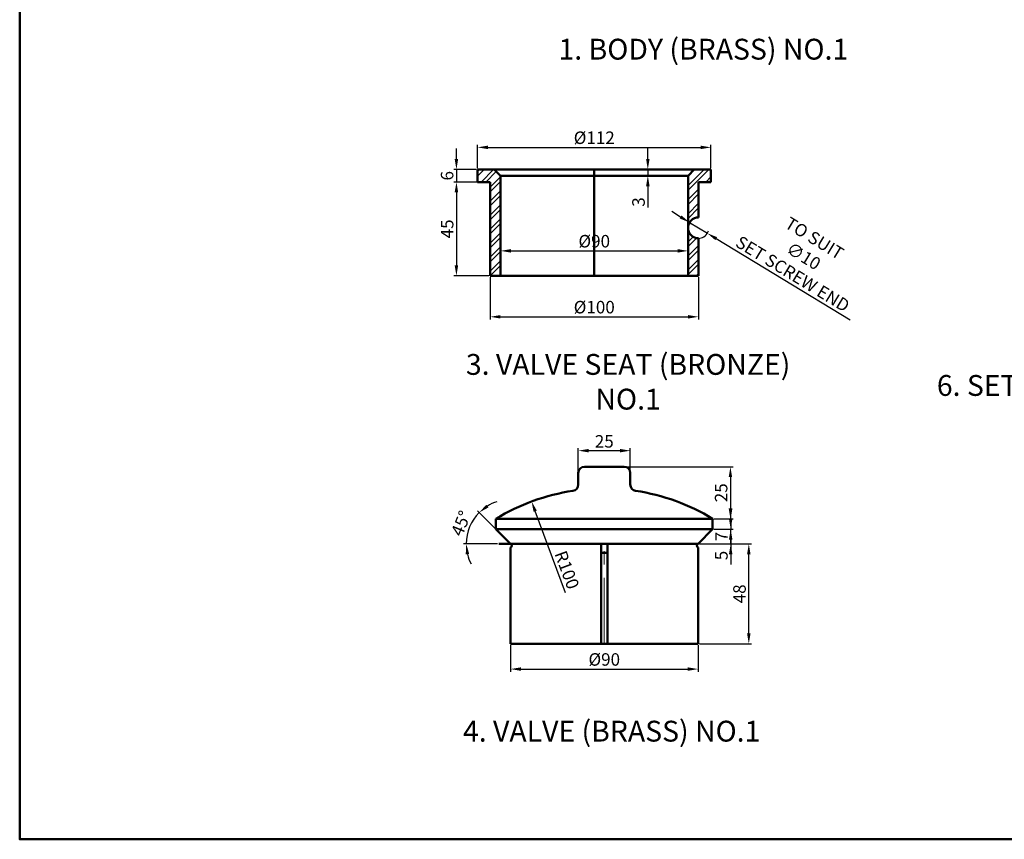
# Model space of a CAD drawing. Units: millimetres. Extents: x -907 to -46, y -312 to 510.
# Tile 1 of 3: x -907 to -434, y -312 to 81. Entities that reach past the tile are written whole.
import ezdxf

# ---------------------------------------------------------------- set-up
doc = ezdxf.new("R2010")
doc.units = ezdxf.units.MM
doc.linetypes.add('CENTER', pattern=[50.8, 31.75, -6.35, 6.35, -6.35])
for name, color, linetype, lineweight in [('M-CNTR', 1, 'CENTER', 18), ('M-DIMS', 2, 'Continuous', 25), ('M-HATC', 8, 'Continuous', 18), ('M-OUTL', 7, 'Continuous', 50), ('M-TEXT', 3, 'Continuous', 25), ('M-TTLB', 7, 'Continuous', 50)]:
    doc.layers.add(name, color=color, linetype=linetype, lineweight=lineweight)
doc.styles.get("Standard").update_dxf_attribs({"font": 'arial.ttf'})
doc.dimstyles.new('ISO-25', dxfattribs={"dimtxt": 6, "dimasz": 5, "dimexe": 1.25, "dimexo": 0.625, "dimtad": 1, "dimtxsty": 'Standard', "dimcen": 2.5, "dimadec": 0, "dimazin": 0, "dimtfac": 1, "dimtmove": 0, "dimatfit": 3, "dimfxl": 1, "dimarcsym": 0})

# ---------------------------------------------------------------- blocks, each defined once
blk = doc.blocks.new('*D24')
at = {"layer": 'Defpoints', "color": 0, "transparency": 16777216}
for p in [(-681.22, -41.73), (-581.22, -41.73), (-581.22, -61.42)]:
    blk.add_point(p, dxfattribs=at)
at = {"layer": 'M-DIMS', "color": 0, "lineweight": -2, "transparency": 16777216}
for p, q in [((-681.22, -42.36), (-681.22, -62.67)), ((-581.22, -42.36), (-581.22, -62.67)), ((-676.22, -61.42), (-586.22, -61.42))]:
    blk.add_line(p, q, dxfattribs=at)
at = {"layer": 'M-DIMS', "color": 0, "transparency": 16777216}
for points in [[(-676.22, -60.58), (-676.22, -62.25), (-681.22, -61.42)], [(-586.22, -60.58), (-586.22, -62.25), (-581.22, -61.42)]]:
    blk.add_solid(points, dxfattribs=at)
at = {"layer": 'M-DIMS', "color": 0, "transparency": 16777216, "insert": (-631.22, -57.56), "char_height": 6, "attachment_point": 5}
blk.add_mtext('%%C100', dxfattribs=at)
blk = doc.blocks.new('*D25')
at = {"layer": 'Defpoints', "color": 0, "transparency": 16777216}
for p in [(-676.22, -21.78), (-586.22, -21.78), (-586.22, -29.78)]:
    blk.add_point(p, dxfattribs=at)
at = {"layer": 'M-DIMS', "color": 0, "lineweight": -2, "transparency": 16777216}
for p, q in [((-676.22, -22.41), (-676.22, -31.03)), ((-586.22, -22.41), (-586.22, -31.03)), ((-671.22, -29.78), (-591.22, -29.78))]:
    blk.add_line(p, q, dxfattribs=at)
at = {"layer": 'M-DIMS', "color": 0, "transparency": 16777216}
for points in [[(-671.22, -28.94), (-671.22, -30.61), (-676.22, -29.78)], [(-591.22, -28.94), (-591.22, -30.61), (-586.22, -29.78)]]:
    blk.add_solid(points, dxfattribs=at)
at = {"layer": 'M-DIMS', "color": 0, "transparency": 16777216, "insert": (-631.22, -25.92), "char_height": 6, "attachment_point": 5}
blk.add_mtext('%%C90', dxfattribs=at)
blk = doc.blocks.new('*D26')
at = {"layer": 'Defpoints', "color": 0, "transparency": 16777216}
for p in [(-606.21, 9.27), (-606.21, 6.27), (-605.51, 6.27)]:
    blk.add_point(p, dxfattribs=at)
at = {"layer": 'M-DIMS', "color": 0, "lineweight": -2, "transparency": 16777216}
for p, q in [((-605.51, 14.27), (-605.51, 19.27)), ((-605.59, 9.27), (-604.26, 9.27)), ((-605.59, 6.27), (-604.26, 6.27)), ((-605.51, 9.27), (-605.51, 6.27)), ((-605.51, 1.27), (-605.51, -8.91))]:
    blk.add_line(p, q, dxfattribs=at)
at = {"layer": 'M-DIMS', "color": 0, "transparency": 16777216}
for points in [[(-606.34, 14.27), (-604.68, 14.27), (-605.51, 9.27)], [(-606.34, 1.27), (-604.68, 1.27), (-605.51, 6.27)]]:
    blk.add_solid(points, dxfattribs=at)
at = {"layer": 'M-DIMS', "color": 0, "transparency": 16777216, "insert": (-609.2, -6.32), "char_height": 6, "attachment_point": 5, "rotation": 90}
blk.add_mtext('3', dxfattribs=at)
blk = doc.blocks.new('*D27')
at = {"layer": 'Defpoints', "color": 0, "transparency": 16777216}
for p in [(-575.22, 19.89), (-687.22, 9.27), (-575.22, 9.27)]:
    blk.add_point(p, dxfattribs=at)
at = {"layer": 'M-DIMS', "color": 0, "lineweight": -2, "transparency": 16777216}
for p, q in [((-687.22, 9.89), (-687.22, 21.14)), ((-682.22, 19.89), (-580.22, 19.89)), ((-575.22, 9.89), (-575.22, 21.14))]:
    blk.add_line(p, q, dxfattribs=at)
at = {"layer": 'M-DIMS', "color": 0, "transparency": 16777216}
for points in [[(-682.22, 20.72), (-682.22, 19.05), (-687.22, 19.89)], [(-580.22, 20.72), (-580.22, 19.05), (-575.22, 19.89)]]:
    blk.add_solid(points, dxfattribs=at)
at = {"layer": 'M-DIMS', "color": 0, "transparency": 16777216, "insert": (-631.22, 23.74), "char_height": 6, "attachment_point": 5}
blk.add_mtext('%%C112', dxfattribs=at)
blk = doc.blocks.new('*D28')
at = {"layer": 'Defpoints', "color": 0, "transparency": 16777216}
for p in [(-687.22, 9.27), (-697.36, 3.27), (-687.22, 3.27)]:
    blk.add_point(p, dxfattribs=at)
at = {"layer": 'M-DIMS', "color": 0, "lineweight": -2, "transparency": 16777216}
for p, q in [((-697.36, 14.27), (-697.36, 19.27)), ((-687.85, 9.27), (-698.61, 9.27)), ((-697.36, 9.27), (-697.36, 3.27)), ((-687.85, 3.27), (-698.61, 3.27)), ((-697.36, -1.73), (-697.36, -6.73))]:
    blk.add_line(p, q, dxfattribs=at)
at = {"layer": 'M-DIMS', "color": 0, "transparency": 16777216}
for points in [[(-698.2, 14.27), (-696.53, 14.27), (-697.36, 9.27)], [(-698.2, -1.73), (-696.53, -1.73), (-697.36, 3.27)]]:
    blk.add_solid(points, dxfattribs=at)
at = {"layer": 'M-DIMS', "color": 0, "transparency": 16777216, "insert": (-701.05, 6.27), "char_height": 6, "attachment_point": 5, "rotation": 90}
blk.add_mtext('6', dxfattribs=at)
blk = doc.blocks.new('*D29')
at = {"layer": 'Defpoints', "color": 0, "transparency": 16777216}
for p in [(-681.22, 3.27), (-697.36, -41.73), (-681.22, -41.73)]:
    blk.add_point(p, dxfattribs=at)
at = {"layer": 'M-DIMS', "color": 0, "lineweight": -2, "transparency": 16777216}
for p, q in [((-681.85, 3.27), (-698.61, 3.27)), ((-697.36, -1.73), (-697.36, -36.73)), ((-681.85, -41.73), (-698.61, -41.73))]:
    blk.add_line(p, q, dxfattribs=at)
at = {"layer": 'M-DIMS', "color": 0, "transparency": 16777216}
for points in [[(-698.2, -1.73), (-696.53, -1.73), (-697.36, 3.27)], [(-698.2, -36.73), (-696.53, -36.73), (-697.36, -41.73)]]:
    blk.add_solid(points, dxfattribs=at)
at = {"layer": 'M-DIMS', "color": 0, "transparency": 16777216, "insert": (-701.04, -19.23), "char_height": 6, "attachment_point": 5, "rotation": 90}
blk.add_mtext('45', dxfattribs=at)
blk = doc.blocks.new('*D30')
at = {"layer": 'Defpoints', "color": 0, "transparency": 16777216}
for p in [(-585.49, -16.13), (-576.95, -21.33)]:
    blk.add_point(p, dxfattribs=at)
at = {"layer": 'M-DIMS', "color": 0, "lineweight": -2, "transparency": 16777216}
for p, q in [((-589.76, -13.53), (-594.04, -10.93)), ((-585.49, -16.13), (-576.95, -21.33)), ((-508.37, -63.06), (-572.68, -23.93))]:
    blk.add_line(p, q, dxfattribs=at)
blk.add_arc((-581.22, -18.73), 5, 277.162, 343.0036, dxfattribs=at)
at = {"layer": 'M-DIMS', "color": 0, "transparency": 16777216}
for points in [[(-589.33, -12.82), (-590.2, -14.25), (-585.49, -16.13)], [(-572.24, -23.22), (-573.11, -24.64), (-576.95, -21.33)]]:
    blk.add_solid(points, dxfattribs=at)
at = {"layer": 'M-DIMS', "color": 0, "transparency": 16777216, "insert": (-531.17, -32.93), "char_height": 6, "attachment_point": 5, "rotation": 328.6797}
blk.add_mtext('TO SUIT\\P∅10\\PSET SCREW END', dxfattribs=at)
blk = doc.blocks.new('*D39')
at = {"layer": 'Defpoints', "color": 0, "transparency": 16777216}
for p in [(-613.91, -125.65), (-638.91, -136.35), (-613.91, -136.35)]:
    blk.add_point(p, dxfattribs=at)
at = {"layer": 'M-DIMS', "color": 0, "lineweight": -2, "transparency": 16777216}
for p, q in [((-638.91, -135.73), (-638.91, -124.4)), ((-633.91, -125.65), (-618.91, -125.65)), ((-613.91, -135.73), (-613.91, -124.4))]:
    blk.add_line(p, q, dxfattribs=at)
at = {"layer": 'M-DIMS', "color": 0, "transparency": 16777216}
for points in [[(-633.91, -124.82), (-633.91, -126.49), (-638.91, -125.65)], [(-618.91, -124.82), (-618.91, -126.49), (-613.91, -125.65)]]:
    blk.add_solid(points, dxfattribs=at)
at = {"layer": 'M-DIMS', "color": 0, "transparency": 16777216, "insert": (-626.41, -121.96), "char_height": 6, "attachment_point": 5}
blk.add_mtext('25', dxfattribs=at)
blk = doc.blocks.new('*D40')
at = {"layer": 'Defpoints', "color": 0, "transparency": 16777216}
for p in [(-616.91, -133.35), (-574.41, -158.35), (-565.88, -158.35)]:
    blk.add_point(p, dxfattribs=at)
at = {"layer": 'M-DIMS', "color": 0, "lineweight": -2, "transparency": 16777216}
for p, q in [((-616.29, -133.35), (-564.63, -133.35)), ((-565.88, -138.35), (-565.88, -153.35)), ((-573.79, -158.35), (-564.63, -158.35))]:
    blk.add_line(p, q, dxfattribs=at)
at = {"layer": 'M-DIMS', "color": 0, "transparency": 16777216}
for points in [[(-566.71, -138.35), (-565.04, -138.35), (-565.88, -133.35)], [(-566.71, -153.35), (-565.04, -153.35), (-565.88, -158.35)]]:
    blk.add_solid(points, dxfattribs=at)
at = {"layer": 'M-DIMS', "color": 0, "transparency": 16777216, "insert": (-569.56, -145.85), "char_height": 6, "attachment_point": 5, "rotation": 90}
blk.add_mtext('25', dxfattribs=at)
blk = doc.blocks.new('*D41')
at = {"layer": 'Defpoints', "color": 0, "transparency": 16777216}
for p in [(-574.41, -158.35), (-574.41, -163.35), (-565.75, -163.35)]:
    blk.add_point(p, dxfattribs=at)
at = {"layer": 'M-DIMS', "color": 0, "lineweight": -2, "transparency": 16777216}
for p, q in [((-565.75, -153.35), (-565.75, -148.35)), ((-573.79, -158.35), (-564.5, -158.35)), ((-565.75, -158.35), (-565.75, -163.35)), ((-573.79, -163.35), (-564.5, -163.35)), ((-565.75, -168.35), (-565.75, -178.58))]:
    blk.add_line(p, q, dxfattribs=at)
at = {"layer": 'M-DIMS', "color": 0, "transparency": 16777216}
for points in [[(-566.58, -153.35), (-564.91, -153.35), (-565.75, -158.35)], [(-566.58, -168.35), (-564.91, -168.35), (-565.75, -163.35)]]:
    blk.add_solid(points, dxfattribs=at)
at = {"layer": 'M-DIMS', "color": 0, "transparency": 16777216, "insert": (-569.42, -175.97), "char_height": 6, "attachment_point": 5, "rotation": 90}
blk.add_mtext('5', dxfattribs=at)
blk = doc.blocks.new('*D42')
at = {"layer": 'Defpoints', "color": 0, "transparency": 16777216}
for p in [(-574.41, -163.35), (-565.75, -163.35), (-581.41, -170.35)]:
    blk.add_point(p, dxfattribs=at)
at = {"layer": 'M-DIMS', "color": 0, "lineweight": -2, "transparency": 16777216}
for p, q in [((-565.75, -158.35), (-565.75, -153.35)), ((-573.79, -163.35), (-564.5, -163.35)), ((-565.75, -170.35), (-565.75, -163.35)), ((-580.79, -170.35), (-564.5, -170.35)), ((-565.75, -175.35), (-565.75, -180.35))]:
    blk.add_line(p, q, dxfattribs=at)
at = {"layer": 'M-DIMS', "color": 0, "transparency": 16777216}
for points in [[(-566.58, -158.35), (-564.91, -158.35), (-565.75, -163.35)], [(-566.58, -175.35), (-564.91, -175.35), (-565.75, -170.35)]]:
    blk.add_solid(points, dxfattribs=at)
at = {"layer": 'M-DIMS', "color": 0, "transparency": 16777216, "insert": (-569.37, -166.85), "char_height": 6, "attachment_point": 5, "rotation": 90}
blk.add_mtext('7', dxfattribs=at)
blk = doc.blocks.new('*D43')
at = {"layer": 'Defpoints', "color": 0, "transparency": 16777216}
for p in [(-689.81, -159.73), (-678.41, -163.35), (-676.96, -170.35), (-667.77, -173.99), (-581.41, -170.35)]:
    blk.add_point(p, dxfattribs=at)
at = {"layer": 'M-DIMS', "color": 0, "lineweight": -2, "transparency": 16777216}
for p, q in [((-678.85, -162.91), (-687.32, -154.45)), ((-677.59, -170.35), (-693.9, -170.35))]:
    blk.add_line(p, q, dxfattribs=at)
for start, end in [(107.9705, 121.4873), (135.004, 180), (193.5168, 207.0335)]:
    blk.add_arc((-671.41, -170.35), 21.24, start, end, dxfattribs=at)
at = {"layer": 'M-DIMS', "color": 0, "transparency": 16777216}
for points in [[(-681.99, -152.89), (-683.02, -151.58), (-686.43, -155.33)], [(-692.89, -175.42), (-691.24, -175.22), (-692.65, -170.35)]]:
    blk.add_solid(points, dxfattribs=at)
at = {"layer": 'M-DIMS', "color": 0, "transparency": 16777216, "insert": (-694.43, -160.82), "char_height": 6, "attachment_point": 5, "rotation": 67.502}
blk.add_mtext('45°', dxfattribs=at)
blk = doc.blocks.new('*D46')
at = {"layer": 'Defpoints', "color": 0, "transparency": 16777216}
for p in [(-671.41, -218.35), (-581.41, -218.35), (-581.41, -230.46)]:
    blk.add_point(p, dxfattribs=at)
at = {"layer": 'M-DIMS', "color": 0, "lineweight": -2, "transparency": 16777216}
for p, q in [((-671.41, -218.98), (-671.41, -231.71)), ((-581.41, -218.98), (-581.41, -231.71)), ((-666.41, -230.46), (-586.41, -230.46))]:
    blk.add_line(p, q, dxfattribs=at)
at = {"layer": 'M-DIMS', "color": 0, "transparency": 16777216}
for points in [[(-666.41, -229.63), (-666.41, -231.3), (-671.41, -230.46)], [(-586.41, -229.63), (-586.41, -231.3), (-581.41, -230.46)]]:
    blk.add_solid(points, dxfattribs=at)
at = {"layer": 'M-DIMS', "color": 0, "transparency": 16777216, "insert": (-626.41, -226.61), "char_height": 6, "attachment_point": 5}
blk.add_mtext('%%C90', dxfattribs=at)
blk = doc.blocks.new('*D47')
at = {"layer": 'Defpoints', "color": 0, "transparency": 16777216}
for p in [(-661.29, -150.05), (-626.41, -243.77)]:
    blk.add_point(p, dxfattribs=at)
at = {"layer": 'M-DIMS', "color": 0, "lineweight": -2, "transparency": 16777216}
blk.add_line((-644.97, -193.9), (-659.54, -154.73), dxfattribs=at)
at = {"layer": 'M-DIMS', "color": 0, "transparency": 16777216}
blk.add_solid([(-658.76, -154.44), (-660.32, -155.02), (-661.29, -150.05)], dxfattribs=at)
at = {"layer": 'M-DIMS', "color": 0, "transparency": 16777216, "insert": (-645.04, -183.13), "char_height": 6, "attachment_point": 5, "rotation": 290.4115}
blk.add_mtext('R100', dxfattribs=at)
blk = doc.blocks.new('*D48')
at = {"layer": 'Defpoints', "color": 0, "transparency": 16777216}
for p in [(-581.41, -170.35), (-557.05, -170.35), (-581.41, -218.35)]:
    blk.add_point(p, dxfattribs=at)
at = {"layer": 'M-DIMS', "color": 0, "lineweight": -2, "transparency": 16777216}
for p, q in [((-580.79, -170.35), (-555.8, -170.35)), ((-557.05, -213.35), (-557.05, -175.35)), ((-580.79, -218.35), (-555.8, -218.35))]:
    blk.add_line(p, q, dxfattribs=at)
at = {"layer": 'M-DIMS', "color": 0, "transparency": 16777216}
for points in [[(-557.89, -175.35), (-556.22, -175.35), (-557.05, -170.35)], [(-557.89, -213.35), (-556.22, -213.35), (-557.05, -218.35)]]:
    blk.add_solid(points, dxfattribs=at)
at = {"layer": 'M-DIMS', "color": 0, "transparency": 16777216, "insert": (-560.74, -194.35), "char_height": 6, "attachment_point": 5, "rotation": 90}
blk.add_mtext('48', dxfattribs=at)

msp = doc.modelspace()

# ---------------------------------------------------------------- hatches: boundary and pattern name
at = {"layer": 'M-HATC'}
h = msp.add_hatch(dxfattribs=at)
h.set_pattern_fill('ANSI32', color=256, scale=0.5)
h.set_pattern_definition([(45, (-1179.6843, -255.1714), (-3.367596, 3.367596), []), (45, (-1177.4392, -255.1714), (-3.367596, 3.367596), [])])
h.paths.add_polyline_path([(-676.2209, 6.2685), (-679.2209, 9.2685), (-687.2209, 9.2685), (-687.2209, 3.2685), (-681.2209, 3.2685), (-681.2209, -41.7315), (-676.2209, -41.7315)])
h.paths.add_polyline_path([(-581.2209, -23.7315, -0.41421356), (-586.2209, -18.7315), (-586.2209, -41.7315), (-581.2209, -41.7315)])
h.paths.add_polyline_path([(-581.2209, 3.2685), (-575.2209, 3.2685), (-575.2209, 9.2685), (-583.2209, 9.2685), (-586.2209, 6.2685), (-586.2209, -18.7315, -0.41421356), (-581.2209, -13.7315)])

# ---------------------------------------------------------------- linework, layer by layer
at = {"layer": 'M-CNTR'}
msp.add_line((-626.411, -218.3522), (-626.411, -170.3522), dxfattribs=at)
at = {"layer": 'M-OUTL'}
for p, q in [((-575.2209, 9.2685), (-687.2209, 9.2685)), ((-687.2209, 9.2685), (-687.2209, 3.2685)), ((-676.2209, 6.2685), (-679.2209, 9.2685)), ((-676.2209, -41.7315), (-676.2209, 6.2685)), ((-586.2209, 6.2685), (-676.2209, 6.2685)), ((-631.2209, -41.7315), (-631.2209, 9.2685)), ((-586.2209, 6.2685), (-583.2209, 9.2685)), ((-586.2209, -41.7315), (-586.2209, 6.2685)), ((-575.2209, 9.2685), (-575.2209, 3.2685)), ((-687.2209, 3.2685), (-681.2209, 3.2685)), ((-681.2209, -41.7315), (-681.2209, 3.2685)), ((-575.2209, 3.2685), (-581.2209, 3.2685)), ((-581.2209, -13.7315), (-581.2209, 3.2685)), ((-581.2209, -41.7315), (-581.2209, -23.7315)), ((-681.2209, -41.7315), (-581.2209, -41.7315)), ((-638.911, -141.9412), (-638.911, -136.3522)), ((-616.911, -133.3522), (-635.911, -133.3522)), ((-613.911, -141.9412), (-613.911, -136.3522)), ((-574.41, -158.3522), (-678.412, -158.3522)), ((-678.412, -158.3522), (-678.412, -163.3522)), ((-574.41, -163.3522), (-574.41, -158.3522)), ((-671.411, -170.3522), (-678.412, -163.3522)), ((-678.412, -163.3522), (-574.41, -163.3522)), ((-581.411, -170.3522), (-574.41, -163.3522)), ((-581.411, -170.3522), (-676.9606, -170.3522)), ((-671.411, -218.3522), (-671.411, -172.0956)), ((-627.911, -218.3522), (-627.911, -170.3522)), ((-627.911, -174.7332), (-624.911, -174.7332)), ((-624.911, -218.3522), (-624.911, -170.3522)), ((-581.411, -218.3522), (-581.411, -172.0956)), ((-671.411, -218.3522), (-581.411, -218.3522))]:
    msp.add_line(p, q, dxfattribs=at)
for centre, radius, start, end in [((-581.2209, -18.7315), 5, 90, 270), ((-635.911, -136.3522), 3, 90, 180), ((-616.911, -136.3522), 3, 0, 90), ((-626.411, -243.7683), 100, 98.655059, 121.332911), ((-641.911, -141.9412), 3, 278.655059, 0), ((-610.911, -141.9412), 3, 180, 261.344941), ((-626.411, -243.7683), 100, 58.667089, 81.344941), ((-671.8024, -171.2239), 0.9555, 294.178906, 65.821094), ((-581.0196, -171.2239), 0.9555, 114.178906, 245.821094)]:
    msp.add_arc(centre, radius, start, end, dxfattribs=at)
at = {"layer": 'M-TTLB'}
msp.add_lwpolyline([(-906.9397, 509.9283), (-45.5255, 509.9283), (-45.5255, -312.1438), (-906.9397, -312.1438)], close=True, dxfattribs=at)

# ---------------------------------------------------------------- texts
at = {"layer": 'M-TEXT', "char_height": 10, "attachment_point": 1}
for s, insert in [('1. BODY (BRASS) NO.1 ', (-648.3572, 72.0056)), ('\\pxqc;3. VALVE SEAT (BRONZE) NO.1 ', (-704.3268, -79.2602)), ('\\pxqc;6. SET SCREW (MILD STEEL) NO.1 ', (-469.0108, -89.3586)), ('4. VALVE (BRASS) NO.1 ', (-694.2223, -255.2533))]:
    msp.add_mtext_dynamic_manual_height_columns(s, width=178.714279, gutter_width=12.5, heights=[0], dxfattribs=dict(at, insert=insert))

# ---------------------------------------------------------------- dimensions: what is measured, and where the dimension line sits
at = {"layer": 'M-DIMS'}
for base, p1, p2, picture, middle in [((-575.2209, 19.8865), (-687.2209, 9.2685), (-575.2209, 9.2685), '*D27', (-631.2209, 23.7427)), ((-586.2209, -29.7754), (-676.2209, -21.7836), (-586.2209, -21.7836), '*D25', (-631.2209, -25.9191)), ((-581.2209, -61.4163), (-681.2209, -41.7315), (-581.2209, -41.7315), '*D24', (-631.2209, -57.5601)), ((-581.411, -230.464), (-671.411, -218.3522), (-581.411, -218.3522), '*D46', (-626.411, -226.6077))]:
    dim = msp.add_linear_dim(base=base, p1=p1, p2=p2, text='%%C<>', dimstyle='ISO-25', override={"dimclrd": 0, "dimclre": 0, "dimclrt": 0}, dxfattribs=at)
    dim.commit()
    dim.dimension.update_dxf_attribs({"geometry": picture, "text_midpoint": middle})
for base, p1, p2, picture, middle in [((-697.3639, 3.2685), (-687.2209, 9.2685), (-687.2209, 3.2685), '*D28', (-701.0523, 6.2685)), ((-605.5084, 6.2685), (-606.212, 9.2685), (-606.212, 6.2685), '*D26', (-609.1989, -6.321)), ((-697.3639, -41.7315), (-681.2209, 3.2685), (-681.2209, -41.7315), '*D29', (-701.04, -19.2315)), ((-565.8758, -158.3522), (-616.911, -133.3522), (-574.41, -158.3522), '*D40', (-569.5643, -145.8522)), ((-565.7473, -163.3522), (-574.41, -158.3522), (-574.41, -163.3522), '*D41', (-569.4234, -175.9663)), ((-565.7473, -163.3522), (-581.411, -170.3522), (-574.41, -163.3522), '*D42', (-569.3723, -166.8522))]:
    dim = msp.add_linear_dim(base=base, p1=p1, p2=p2, angle=90, dimstyle='ISO-25', override={"dimclrd": 0, "dimclre": 0, "dimclrt": 0}, dxfattribs=at)
    dim.commit()
    dim.dimension.update_dxf_attribs({"geometry": picture, "text_midpoint": middle})
dim = msp.add_diameter_dim_2p(p1=(-585.4923, -16.1323), p2=(-576.9495, -21.3306), text='TO SUIT\\P<>\\PSET SCREW END', dimstyle='ISO-25', override={"dimclrd": 0, "dimclre": 0, "dimclrt": 0}, dxfattribs=at)
dim.commit()
dim.dimension.update_dxf_attribs({"geometry": '*D30', "text_midpoint": (-531.1656, -32.9293)})
dim = msp.add_linear_dim(base=(-613.911, -125.6517), p1=(-638.911, -136.3522), p2=(-613.911, -136.3522), dimstyle='ISO-25', override={"dimclrd": 0, "dimclre": 0, "dimclrt": 0}, dxfattribs=at)
dim.commit()
dim.dimension.update_dxf_attribs({"geometry": '*D39', "text_midpoint": (-626.411, -121.9633)})
dim = msp.add_angular_dim_2l(base=(-689.809, -159.7313), line1=((-581.411, -170.3522), (-676.9606, -170.3522)), line2=((-667.7703, -173.9924), (-678.412, -163.3522)), dimstyle='ISO-25', override={"dimclrd": 0, "dimclre": 0, "dimclrt": 0}, dxfattribs=at)
dim.commit()
dim.dimension.update_dxf_attribs({"geometry": '*D43', "text_midpoint": (-694.4342, -160.8167)})
dim = msp.add_radius_dim(center=(-626.411, -243.7683), mpoint=(-661.2869, -150.047), dimstyle='ISO-25', override={"dimclrd": 0, "dimclre": 0, "dimclrt": 0}, dxfattribs=at)
dim.commit()
dim.dimension.update_dxf_attribs({"geometry": '*D47', "text_midpoint": (-648.4965, -184.4185), "dimtype": 164})
dim = msp.add_linear_dim(base=(-557.0527, -170.3522), p1=(-581.411, -218.3522), p2=(-581.411, -170.3522), angle=90, dimstyle='ISO-25', override={"dimclrd": 0, "dimclre": 0, "dimclrt": 0}, dxfattribs=at)
dim.commit()
dim.dimension.update_dxf_attribs({"geometry": '*D48', "text_midpoint": (-557.0527, -194.3522), "dimtype": 160})

doc.saveas('drawing.dxf')
